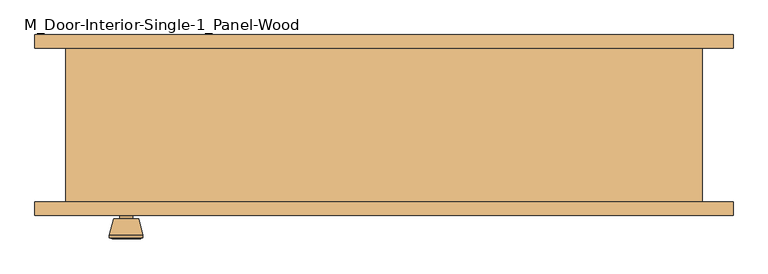
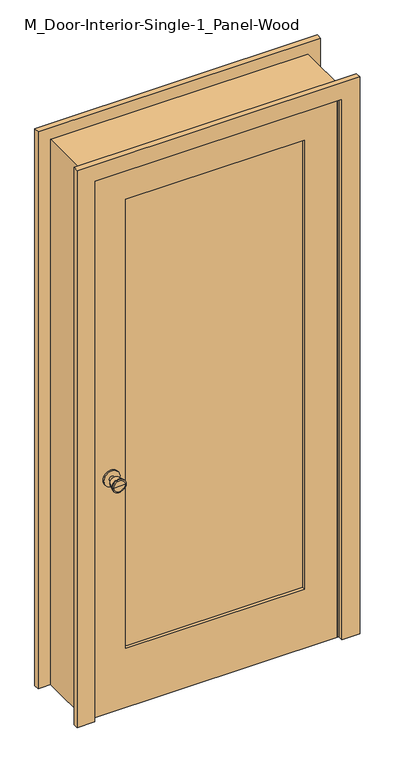
"""IFC4 building model written with IfcOpenShell, lengths in millimetres: door geometry, M_Door-Interior-Single-1_Panel-Wood."""

from ifc_helpers import new_model, si_unit, point, frame, frame_2d, origin, place, context, project, spatial, polyline, circle_curve, trimmed, segment, composite_curve, outline, extrude, faceted_brep, source, transform, mapped, element, save
from ifc_brep_helpers import plane_surface, cylinder_surface, revolved_surface, advanced_brep


def m_door_interior_single_1_panel_wood_b1ec41f7(model_context):
    return source(origin(), model_context, "Body", "SolidModel", [
        advanced_brep(
        [(-385.0, -70.825, 914.4), (-395.0, -70.825, 914.4), (-375.0, -70.825, 914.4), (-364.5241324, -21.825, 914.4), (-405.4758676, -21.825, 914.4), (-385.0, -21.825, 914.4), (-360.0, -23.6528681, 914.4), (-410.0, -23.6528681, 914.4), (-360.0, -27.1165463, 914.4), (-410.0, -27.1165463, 914.4), (-366.363764, -51.825, 914.4), (-403.636236, -51.825, 914.4), (-375.0, -51.825, 914.4), (-395.0, -51.825, 914.4)],
        [
            (0, 1),
            (1, 2, circle_curve(frame((-385.0, -70.825, 914.4), z_axis=(0.0, -1.0, 0.0), x_axis=(-1.0, 0.0, 0.0)), 10.0)),
            (2, 0),
            (2, 1, circle_curve(frame((-385.0, -70.825, 914.4), z_axis=(0.0, -1.0, 0.0), x_axis=(-1.0, 0.0, 0.0)), 10.0)),
            (3, 4, circle_curve(frame((-385.0, -21.825, 914.4), z_axis=(0.0, 1.0, 0.0), x_axis=(-1.0, 0.0, 0.0)), 20.4758676)),
            (4, 5),
            (5, 3),
            (4, 3, circle_curve(frame((-385.0, -21.825, 914.4), z_axis=(0.0, 1.0, 0.0), x_axis=(-1.0, 0.0, 0.0)), 20.4758676)),
            (6, 7, circle_curve(frame((-385.0, -23.6528681, 914.4), z_axis=(0.0, 1.0, 0.0), x_axis=(-1.0, 0.0, 0.0)), 25.0)),
            (7, 4),
            (3, 6),
            (7, 6, circle_curve(frame((-385.0, -23.6528681, 914.4), z_axis=(0.0, 1.0, 0.0), x_axis=(-1.0, 0.0, 0.0)), 25.0)),
            (8, 9, circle_curve(frame((-385.0, -27.1165463, 914.4), z_axis=(0.0, 1.0, 0.0), x_axis=(-1.0, 0.0, 0.0)), 25.0)),
            (9, 7),
            (6, 8),
            (9, 8, circle_curve(frame((-385.0, -27.1165463, 914.4), z_axis=(0.0, 1.0, 0.0), x_axis=(-1.0, 0.0, 0.0)), 25.0)),
            (10, 11, circle_curve(frame((-385.0, -51.825, 914.4), z_axis=(0.0, 1.0, 0.0), x_axis=(-1.0, 0.0, 0.0)), 18.636236)),
            (11, 9),
            (8, 10),
            (11, 10, circle_curve(frame((-385.0, -51.825, 914.4), z_axis=(0.0, 1.0, 0.0), x_axis=(-1.0, 0.0, 0.0)), 18.636236)),
            (12, 13, circle_curve(frame((-385.0, -51.825, 914.4), z_axis=(0.0, 1.0, 0.0), x_axis=(-1.0, 0.0, 0.0)), 10.0)),
            (13, 11),
            (10, 12),
            (13, 12, circle_curve(frame((-385.0, -51.825, 914.4), z_axis=(0.0, 1.0, 0.0), x_axis=(-1.0, 0.0, 0.0)), 10.0)),
            (1, 13),
            (12, 2),
        ],
        [
            plane_surface(frame((-385.0, -70.825, 914.4), z_axis=(0.0, -1.0, 0.0), x_axis=(-1.0, 0.0, 0.0))),
            plane_surface(frame((-385.0, -21.825, 914.4), z_axis=(0.0, 1.0, 0.0), x_axis=(-1.0, 0.0, 0.0))),
            revolved_surface(polyline([(-405.4758676, -21.825, 914.4), (-410.0, -23.6528681, 914.4)]), (-385.0, -70.825, 914.4), (0.0, -1.0, 0.0)),
            cylinder_surface(frame((-385.0, -70.825, 914.4), z_axis=(0.0, -1.0, 0.0), x_axis=(-1.0, 0.0, 0.0)), 25.0),
            revolved_surface(polyline([(-410.0, -27.1165463, 914.4), (-403.636236, -51.825, 914.4)]), (-385.0, -70.825, 914.4), (0.0, -1.0, 0.0)),
            plane_surface(frame((-385.0, -51.825, 914.4), z_axis=(0.0, -1.0, 0.0), x_axis=(-1.0, 0.0, 0.0))),
            cylinder_surface(frame((-385.0, -70.825, 914.4), z_axis=(0.0, -1.0, 0.0), x_axis=(-1.0, 0.0, 0.0)), 10.0),
        ],
        [
            (0, [[1, 2, 3]]),
            (0, [[-3, 4, -1]]),
            (1, [[5, 6, 7]]),
            (1, [[8, -7, -6]]),
            (2, [[9, 10, -5, 11]]),
            (2, [[12, -11, -8, -10]]),
            (3, [[13, 14, -9, 15]]),
            (3, [[16, -15, -12, -14]]),
            (4, [[17, 18, -13, 19]]),
            (4, [[20, -19, -16, -18]]),
            (5, [[21, 22, -17, 23]]),
            (5, [[24, -23, -20, -22]]),
            (6, [[-2, 25, -21, 26]]),
            (6, [[-4, -26, -24, -25]]),
        ],
    ),
        extrude(outline(composite_curve([segment(trimmed(circle_curve(frame_2d((914.4, -385.0)), 30.0), [point((914.4, -415.0))], [point((914.4, -355.0))], False, "CARTESIAN"), True, "CONTINUOUS"), segment(trimmed(circle_curve(frame_2d((914.4, -385.0)), 30.0), [point((914.4, -355.0))], [point((914.4, -415.0))], False, "CARTESIAN"), True, "CONTINUOUS")], self_intersect=False)), frame((0.0, -76.825, 0.0), z_axis=(0.0, 1.0, 0.0), x_axis=(0.0, 0.0, 1.0)), (0.0, 0.0, 1.0), 6.0),
        advanced_brep(
        [(-385.0, -117.825, 914.4), (-375.0, -117.825, 914.4), (-395.0, -117.825, 914.4), (-364.5241324, -166.825, 914.4), (-385.0, -166.825, 914.4), (-405.4758676, -166.825, 914.4), (-360.0, -164.9971319, 914.4), (-410.0, -164.9971319, 914.4), (-360.0, -161.5334537, 914.4), (-410.0, -161.5334537, 914.4), (-366.363764, -136.825, 914.4), (-403.636236, -136.825, 914.4), (-375.0, -136.825, 914.4), (-395.0, -136.825, 914.4)],
        [
            (0, 1),
            (1, 2, circle_curve(frame((-385.0, -117.825, 914.4), z_axis=(0.0, 1.0, 0.0), x_axis=(-1.0, 0.0, 0.0)), 10.0)),
            (2, 0),
            (2, 1, circle_curve(frame((-385.0, -117.825, 914.4), z_axis=(0.0, 1.0, 0.0), x_axis=(-1.0, 0.0, 0.0)), 10.0)),
            (3, 4),
            (4, 5),
            (5, 3, circle_curve(frame((-385.0, -166.825, 914.4), z_axis=(0.0, -1.0, 0.0), x_axis=(-1.0, 0.0, 0.0)), 20.4758676)),
            (3, 5, circle_curve(frame((-385.0, -166.825, 914.4), z_axis=(0.0, -1.0, 0.0), x_axis=(-1.0, 0.0, 0.0)), 20.4758676)),
            (6, 3),
            (5, 7),
            (7, 6, circle_curve(frame((-385.0, -164.9971319, 914.4), z_axis=(0.0, -1.0, 0.0), x_axis=(-1.0, 0.0, 0.0)), 25.0)),
            (6, 7, circle_curve(frame((-385.0, -164.9971319, 914.4), z_axis=(0.0, -1.0, 0.0), x_axis=(-1.0, 0.0, 0.0)), 25.0)),
            (8, 6),
            (7, 9),
            (9, 8, circle_curve(frame((-385.0, -161.5334537, 914.4), z_axis=(0.0, -1.0, 0.0), x_axis=(-1.0, 0.0, 0.0)), 25.0)),
            (8, 9, circle_curve(frame((-385.0, -161.5334537, 914.4), z_axis=(0.0, -1.0, 0.0), x_axis=(-1.0, 0.0, 0.0)), 25.0)),
            (10, 8),
            (9, 11),
            (11, 10, circle_curve(frame((-385.0, -136.825, 914.4), z_axis=(0.0, -1.0, 0.0), x_axis=(-1.0, 0.0, 0.0)), 18.636236)),
            (10, 11, circle_curve(frame((-385.0, -136.825, 914.4), z_axis=(0.0, -1.0, 0.0), x_axis=(-1.0, 0.0, 0.0)), 18.636236)),
            (12, 10),
            (11, 13),
            (13, 12, circle_curve(frame((-385.0, -136.825, 914.4), z_axis=(0.0, -1.0, 0.0), x_axis=(-1.0, 0.0, 0.0)), 10.0)),
            (12, 13, circle_curve(frame((-385.0, -136.825, 914.4), z_axis=(0.0, -1.0, 0.0), x_axis=(-1.0, 0.0, 0.0)), 10.0)),
            (1, 12),
            (13, 2),
        ],
        [
            plane_surface(frame((-385.0, -117.825, 914.4), z_axis=(0.0, 1.0, 0.0), x_axis=(-1.0, 0.0, 0.0))),
            plane_surface(frame((-385.0, -166.825, 914.4), z_axis=(0.0, -1.0, 0.0), x_axis=(-1.0, 0.0, 0.0))),
            revolved_surface(polyline([(-405.4758676, -166.825, 914.4), (-410.0, -164.9971319, 914.4)]), (-385.0, -117.825, 914.4), (0.0, 1.0, 0.0)),
            cylinder_surface(frame((-385.0, -117.825, 914.4), z_axis=(0.0, 1.0, 0.0), x_axis=(-1.0, 0.0, 0.0)), 25.0),
            revolved_surface(polyline([(-410.0, -161.5334537, 914.4), (-403.636236, -136.825, 914.4)]), (-385.0, -117.825, 914.4), (0.0, 1.0, 0.0)),
            plane_surface(frame((-385.0, -136.825, 914.4), z_axis=(0.0, 1.0, 0.0), x_axis=(-1.0, 0.0, 0.0))),
            cylinder_surface(frame((-385.0, -117.825, 914.4), z_axis=(0.0, 1.0, 0.0), x_axis=(-1.0, 0.0, 0.0)), 10.0),
        ],
        [
            (0, [[1, 2, 3]]),
            (0, [[-3, 4, -1]]),
            (1, [[5, 6, 7]]),
            (1, [[-6, -5, 8]]),
            (2, [[9, -7, 10, 11]]),
            (2, [[-10, -8, -9, 12]]),
            (3, [[13, -11, 14, 15]]),
            (3, [[-14, -12, -13, 16]]),
            (4, [[17, -15, 18, 19]]),
            (4, [[-18, -16, -17, 20]]),
            (5, [[21, -19, 22, 23]]),
            (5, [[-22, -20, -21, 24]]),
            (6, [[25, -23, 26, -2]]),
            (6, [[-26, -24, -25, -4]]),
        ],
    ),
        extrude(outline(composite_curve([segment(trimmed(circle_curve(frame_2d((914.4, -385.0)), 30.0), [point((914.4, -415.0))], [point((914.4, -355.0))], False, "CARTESIAN"), True, "CONTINUOUS"), segment(trimmed(circle_curve(frame_2d((914.4, -385.0)), 30.0), [point((914.4, -355.0))], [point((914.4, -415.0))], False, "CARTESIAN"), True, "CONTINUOUS")], self_intersect=False)), frame((0.0, -117.825, 0.0), z_axis=(0.0, 1.0, 0.0), x_axis=(0.0, 0.0, 1.0)), (0.0, 0.0, 1.0), 6.0),
        faceted_brep([(475.0, -111.825, 0.0), (450.0, -111.825, 0.0), (450.0, -76.825, 0.0), (437.3, -76.825, 0.0), (437.3, -41.9, 0.0), (450.0, -41.9, 0.0), (450.0, 118.175, 0.0), (475.0, 118.175, 0.0), (475.0, 118.175, 2125.0), (475.0, -111.825, 2125.0), (450.0, 118.175, 2100.0), (-450.0, 118.175, 2100.0), (-450.0, 118.175, 0.0), (-475.0, 118.175, 0.0), (-475.0, 118.175, 2125.0), (450.0, -41.9, 2100.0), (437.3, -41.9, 2087.3), (-437.3, -41.9, 2087.3), (-437.3, -41.9, 0.0), (-450.0, -41.9, 0.0), (-450.0, -41.9, 2100.0), (437.3, -76.825, 2087.3), (450.0, -76.825, 2100.0), (-450.0, -76.825, 2100.0), (-450.0, -76.825, 0.0), (-437.3, -76.825, 0.0), (-437.3, -76.825, 2087.3), (450.0, -111.825, 2100.0), (-475.0, -111.825, 2125.0), (-475.0, -111.825, 0.0), (-450.0, -111.825, 0.0), (-450.0, -111.825, 2100.0)], [[[0, 1, 2, 3, 4, 5, 6, 7]], [[7, 8, 9, 0]], [[6, 10, 11, 12, 13, 14, 8, 7]], [[5, 15, 10, 6]], [[4, 16, 17, 18, 19, 20, 15, 5]], [[3, 21, 16, 4]], [[2, 22, 23, 24, 25, 26, 21, 3]], [[1, 27, 22, 2]], [[0, 9, 28, 29, 30, 31, 27, 1]], [[8, 14, 28, 9]], [[15, 20, 11, 10]], [[21, 26, 17, 16]], [[27, 31, 23, 22]], [[29, 13, 12, 19, 18, 25, 24, 30]], [[14, 13, 29, 28]], [[20, 19, 12, 11]], [[26, 25, 18, 17]], [[31, 30, 24, 23]]]),
        extrude(outline(polyline([(2100.0, -450.0), (0.0, -450.0), (0.0, 450.0), (2100.0, 450.0), (2100.0, -450.0)]), holes=[polyline([(1980.0, -330.0), (1980.0, 330.0), (230.0, 330.0), (230.0, -330.0), (1980.0, -330.0)])]), frame((0.0, -111.825, 0.0), z_axis=(0.0, 1.0, 0.0), x_axis=(0.0, 0.0, 1.0)), (0.0, 0.0, 1.0), 35.0),
        extrude(outline(polyline([(330.0, -88.4916667), (330.0, -100.1583333), (-330.0, -100.1583333), (-330.0, -88.4916667), (330.0, -88.4916667)])), frame((0.0, 0.0, 230.0), z_axis=(0.0, 0.0, 1.0), x_axis=(1.0, 0.0, 0.0)), (0.0, 0.0, 1.0), 1750.0),
        extrude(outline(polyline([(0.0, 521.35), (2171.35, 521.35), (2171.35, -521.35), (0.0, -521.35), (0.0, -456.35), (2106.35, -456.35), (2106.35, 456.35), (0.0, 456.35), (0.0, 521.35)])), frame((0.0, -131.825, 0.0), z_axis=(0.0, 1.0, 0.0), x_axis=(0.0, 0.0, 1.0)), (0.0, 0.0, 1.0), 20.0),
        extrude(outline(polyline([(0.0, 521.35), (2171.35, 521.35), (2171.35, -521.35), (0.0, -521.35), (0.0, -456.35), (2106.35, -456.35), (2106.35, 456.35), (0.0, 456.35), (0.0, 521.35)])), frame((0.0, 118.175, 0.0), z_axis=(0.0, 1.0, 0.0), x_axis=(0.0, 0.0, 1.0)), (0.0, 0.0, 1.0), 20.0),
    ])


if __name__ == "__main__":
    model = new_model("IFC4")
    model_context = context("Model", 3, world=origin())
    ifc_project = project(units=[si_unit("LENGTHUNIT", "METRE", prefix="MILLI")], contexts=[model_context])
    site = spatial("IfcSite", under=ifc_project)
    building = spatial("IfcBuilding", under=site)
    placement = place(None, origin())
    m_door_interior_single_1_panel_wood_shape = m_door_interior_single_1_panel_wood_b1ec41f7(model_context)
    element("IfcDoor", 1, ObjectType="M_Door-Interior-Single-1_Panel-Wood", at=placement, inside=building, context=model_context, shape_type="MappedRepresentation", body=[
        mapped(m_door_interior_single_1_panel_wood_shape, transform((0.0, 0.0, 0.0), x_axis=(1.0, 0.0, 0.0), y_axis=(0.0, 1.0, 0.0), z_axis=(0.0, 0.0, 1.0))),
    ])
    save(model, "model.ifc")

# Revit data of these elements
# Type "M_Door-Interior-Single-1_Panel-Wood"
#   Type Mark = "26"
#   Assembly Code = "C1020300"
#   Analytic Construction = "Wooden"
#   Top Rail = 120 mm
#   Thickness = 35 mm
#   Thermal Resistance (R) = 0.455703 (m²·K)/W
#   Swing Angle [instance default] = 90.00°
#   Stiles = 120 mm
#   Rough Width = 950 mm
#   Rough Height = 2125 mm
#   Height = 2100 mm
#   Width = 900 mm
#   Heat Transfer Coefficient (U) = 2.19465 W/(m²·K)
#   Bottom Rail = 230 mm
#   Trim Material = Cherry
#   Panel Material = Cherry
#   Frame Material = Cherry
#   Door Handle Material = Aluminum
#   Visual Light Transmittance = 0
#   Solar Heat Gain Coefficient = 0
#   Wall Closure = (empty or 0)
#   Function = (empty or 0)
# Element 1 (IfcDoor, "M_Door-Interior-Single-1_Panel-Wood")
#   Materials on its faces: "Cherry", "Aluminum"
# Materials
#   "Cherry": class "Wood", colour RGB 154 107 61, transparency 0, Description = "Prunus Serotina", Cost = 0
#   "Aluminum": class "Metal", colour RGB 244 244 244, transparency 0, Description = "Aluminum 6061", Cost = 0
